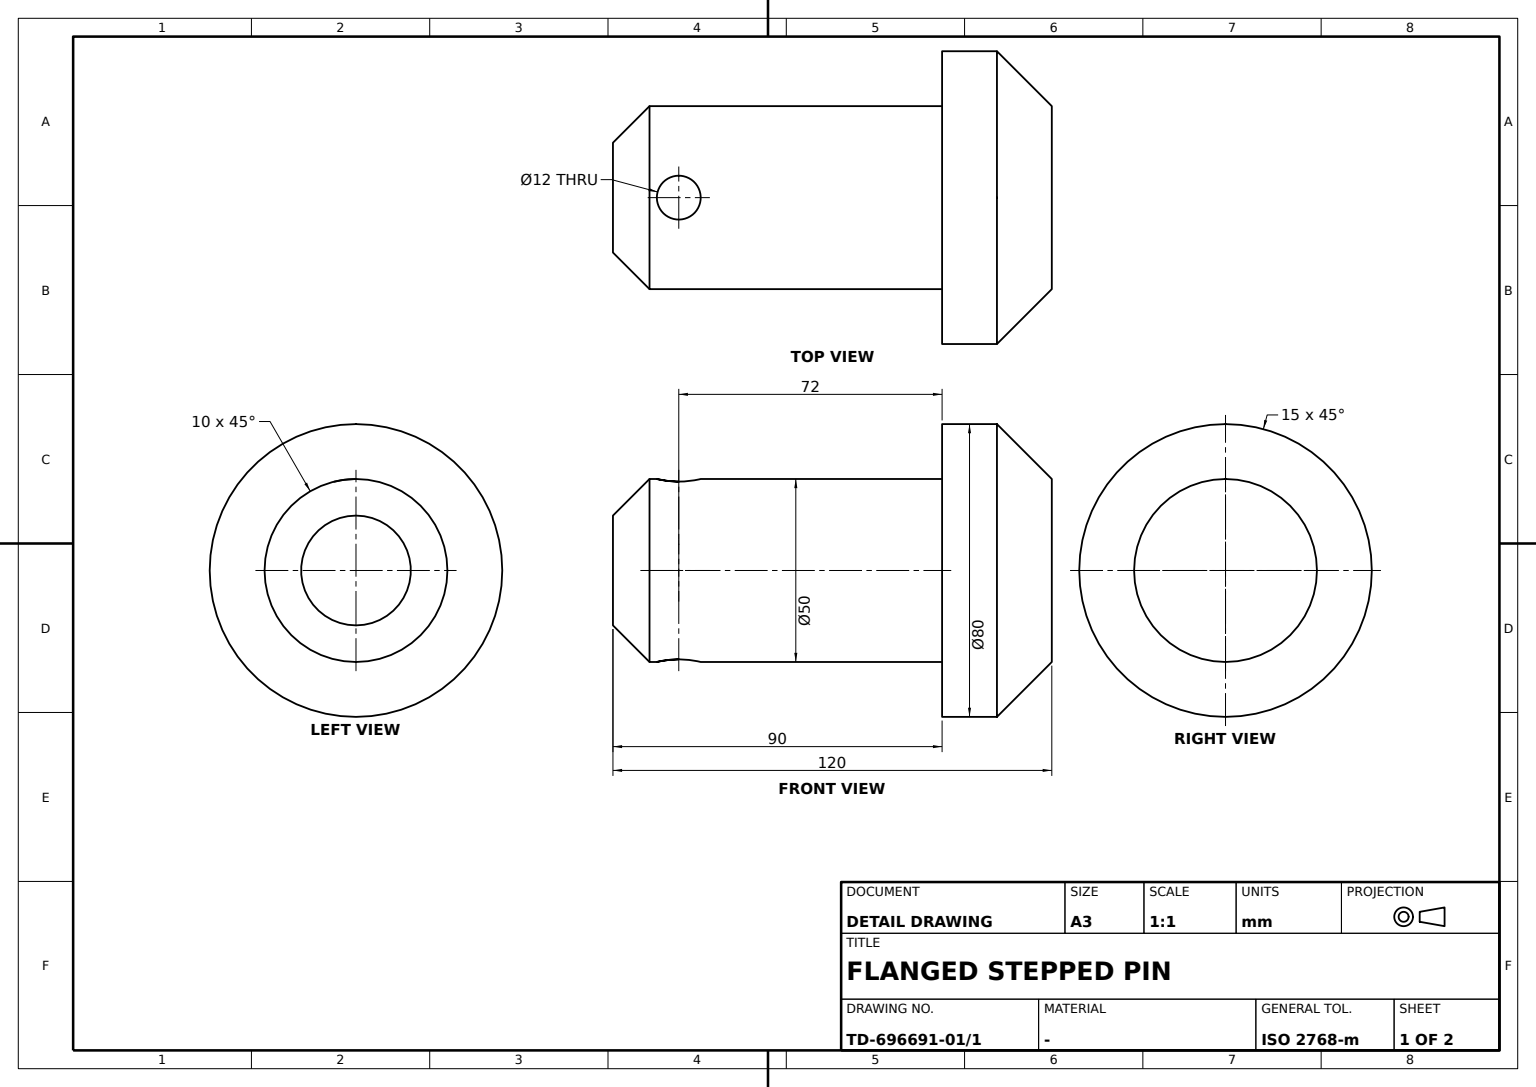
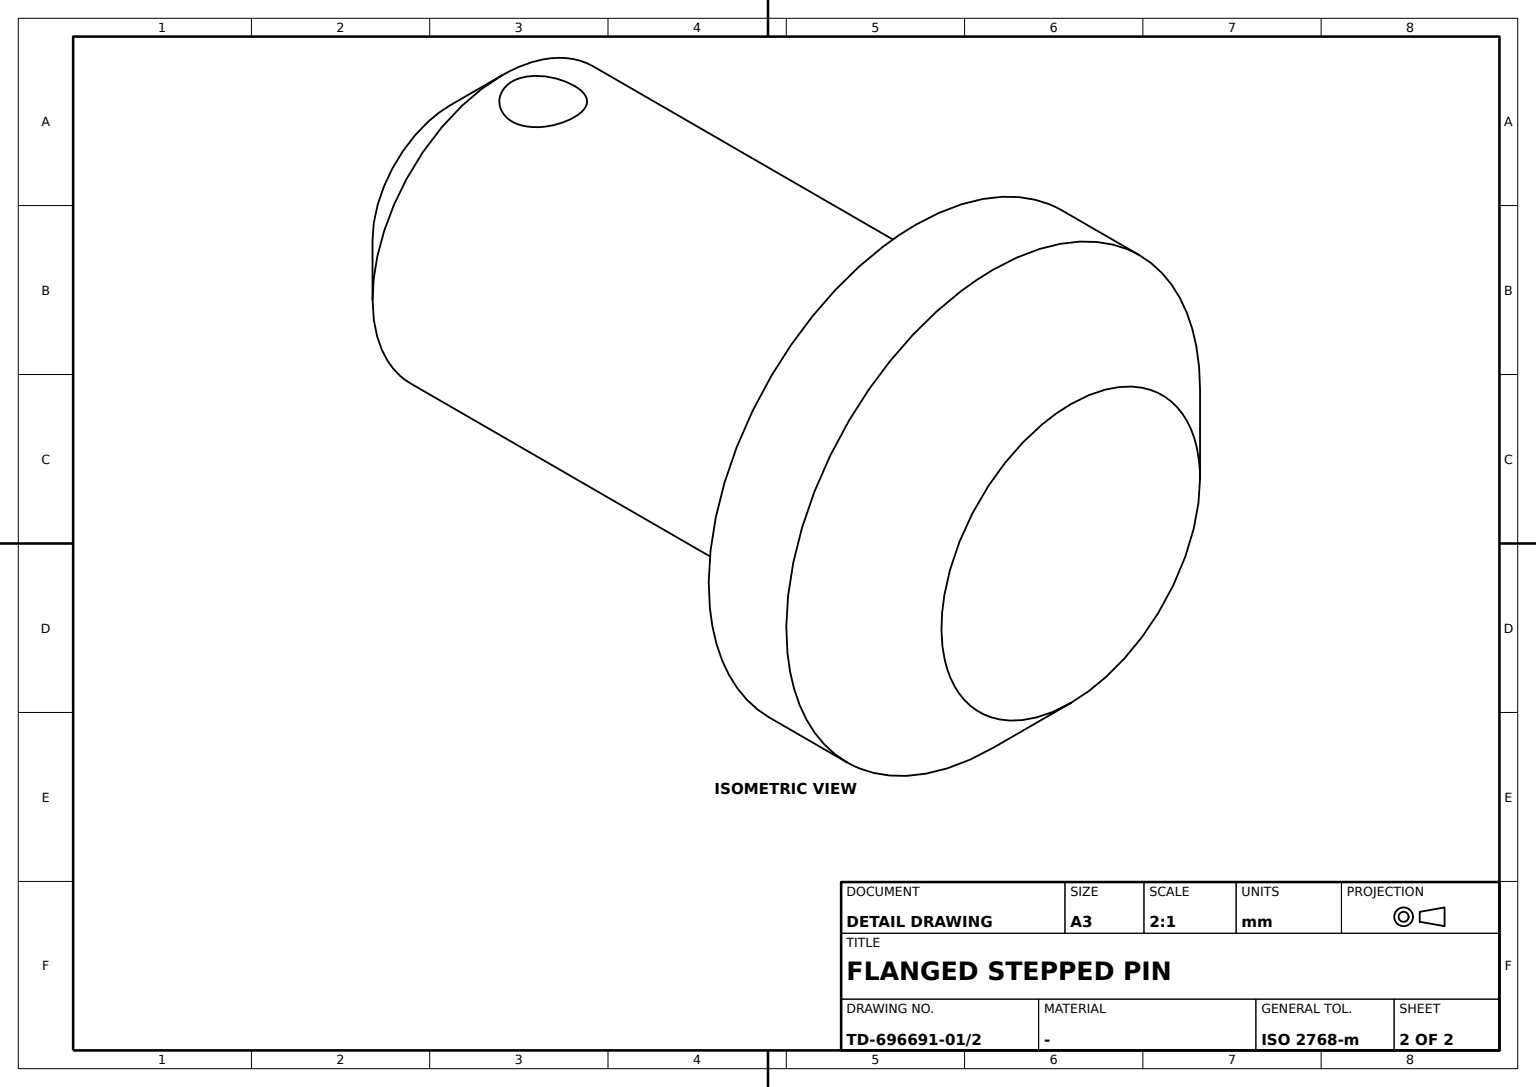
CATIA V5 part; units mm, degrees
sketch "Sketch1" plane through (0, 0, 0) normal (-1, 0, 0) x (0, -1, 0)
  circle A0 centre (0, 0) radius 40
  point P0 (0, 0)
  dimension "radius A0" = 40
  constraint coincidence P0 y-axis
  constraint coincidence origin P0
extrude "Pad1" add sketch "Sketch1" along normal blind 30
sketch "Sketch2" plane through (-30, 0, 0) normal (-1, 0, 0) x (0, -1, 0)
  circle A0 centre (0, 0) radius 25
  dimension "radius A0" = 25
extrude "Pad2" add sketch "Sketch2" along normal blind 90
chamfer "Chamfer1" distance 10 angle 45 1 edges at (-120, 25, 0)
chamfer "Chamfer2" distance 15 angle 45 1 edges at (0, 40, 0)
sketch "Sketch3" plane through (0, 0, 0) normal (0, 0, 1) x (0, 1, 0)
  circle A0 centre (0, 102) radius 6
  point P0 (0, 102)
  line L0 (-40, 30) -> (40, 30) construction
  dimension "radius A0" = 6
  dimension "distance P0 L0" = 72
  constraint coincidence P0 y-axis
extrude "Pocket1" cut sketch "Sketch3" along normal mid plane 180
